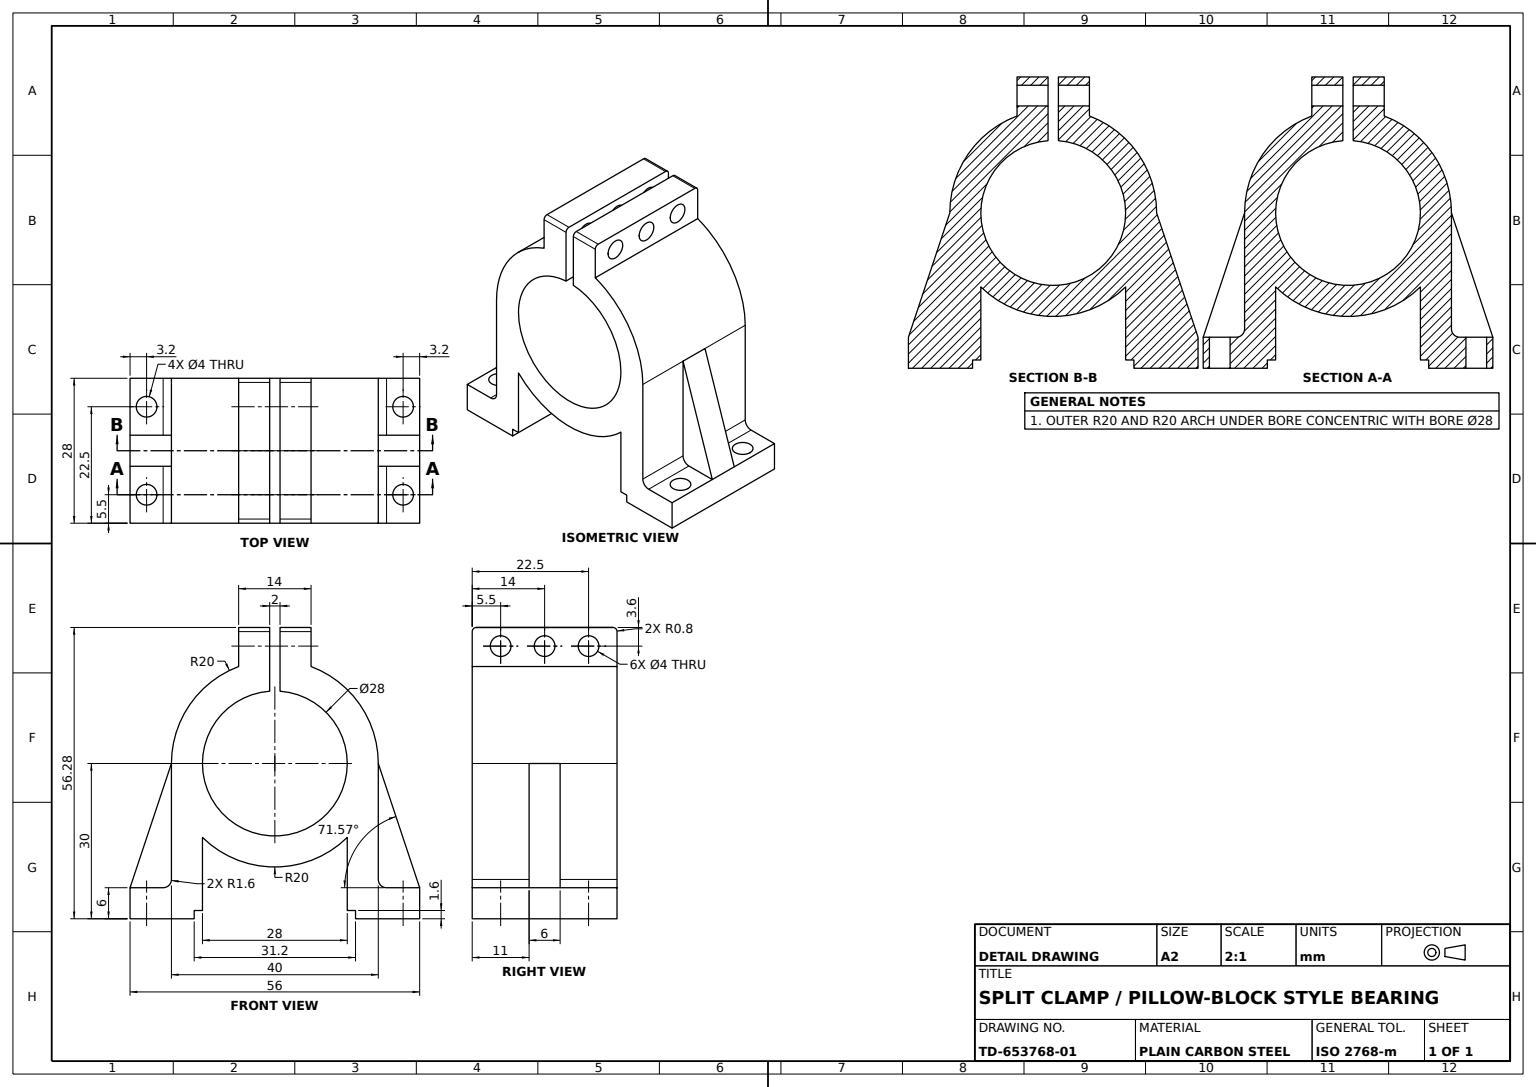
from build123d import *

# Parameters (mm, degrees)
CLAMP_BODY_DEPTH             = 14
CLAMP_BORE_SKETCH_R          = 14
CLAMP_BORE_DEPTH             = 96
CLAMP_LUGS_DEPTH             = 28
SPLIT_SLOT_2MM_DEPTH         = 52
BODY_FILLET_R1_6_A_R         = 1.6
BODY_FILLET_R1_6_B_R         = 1.6
CLAMP_SCREW_HOLES_SKETCH_R   = 2
CLAMP_SCREW_HOLES_3X_DEPTH   = 52
SUPPORT_RIB_1_REACH          = 61.228
SUPPORT_RIB_1_SKETCH_WALL_W  = 145.754223634
SUPPORT_RIB_1_SKETCH_WALL_H  = 6
SUPPORT_RIB_2_REACH          = 61.228
SUPPORT_RIB_2_SKETCH_WALL_W  = 145.754223634
SUPPORT_RIB_2_SKETCH_WALL_H  = 6
BASE_MOUNTING_HOLES_SKETCH_R = 2
BASE_MOUNTING_HOLES_4X_DEPTH = 52
LUG_FILLET_R0_8_A_R          = 0.8
LUG_FILLET_R0_8_B_R          = 0.8
LUG_FILLET_R0_8_C_R          = 0.8
LUG_FILLET_R0_8_D_R          = 0.8


with BuildPart() as part:
    # Clamp Body Profile → Clamp Body (new, symmetric)
    with BuildSketch(Plane.XY):
        with BuildLine():
            Line((20, 24), (20, 0))
            Line((20, 0), (28, 0))
            Line((28, 0), (28, -6))
            Line((28, -6), (15.6, -6))
            Line((15.6, -6), (15.6, -4.4))
            Line((15.6, -4.4), (14, -4.4))
            Line((14, -4.4), (14, 9.717143143))
            ThreePointArc((14, 9.717143143), (0, 4), (-14, 9.717143143))
            Line((-14, 9.717143143), (-14, -4.4))
            Line((-14, -4.4), (-15.6, -4.4))
            Line((-15.6, -4.4), (-15.6, -6))
            Line((-15.6, -6), (-28, -6))
            Line((-28, -6), (-28, 0))
            Line((-28, 0), (-20, 0))
            Line((-20, 0), (-20, 24))
            ThreePointArc((-20, 24), (0, 44), (20, 24))
        make_face()
    extrude(amount=CLAMP_BODY_DEPTH, both=True)

    # Clamp Bore Sketch → Clamp Bore (cut)
    with BuildSketch(Plane.XY.offset(14)):
        with Locations((0, 24)):
            Circle(CLAMP_BORE_SKETCH_R)
    extrude(amount=-CLAMP_BORE_DEPTH, mode=Mode.SUBTRACT)

    # Clamp Lugs Sketch → Clamp Lugs (add)
    with BuildSketch(Plane.XY.offset(14)):
        Polygon((0, 38), (7, 38), (7, 42.734993995), (7, 50.278784028), (-7, 50.278784028), (-7, 38), align=None)
    extrude(amount=-CLAMP_LUGS_DEPTH)

    # Split Slot Sketch → Split Slot 2mm (cut)
    with BuildSketch(Plane.XY.offset(14)):
        Polygon((-1, 37.964240044), (-1, 37.406271495), (1, 37.406271495), (1, 38), (1, 50.278784028), (-1, 50.278784028), align=None)
    extrude(amount=-SPLIT_SLOT_2MM_DEPTH, mode=Mode.SUBTRACT)

    # Body Fillet R1.6 A
    body_fillet_r1_6_a_edges = [part.edges().sort_by_distance(p)[0] for p in [
        (20, 0, 0),
    ]]
    fillet(body_fillet_r1_6_a_edges, radius=BODY_FILLET_R1_6_A_R)

    # Body Fillet R1.6 B
    body_fillet_r1_6_b_edges = [part.edges().sort_by_distance(p)[0] for p in [
        (-20, 0, 0),
    ]]
    fillet(body_fillet_r1_6_b_edges, radius=BODY_FILLET_R1_6_B_R)

    # Clamp Screw Holes Sketch → Clamp Screw Holes 3x (cut)
    with BuildSketch(Plane(origin=(7, 0, 0), x_dir=(0, 0, -1), z_dir=(1, 0, 0))):
        with Locations((8.5, 46.678784028)):
            Circle(CLAMP_SCREW_HOLES_SKETCH_R)
        with Locations((-8.5, 46.678784028)):
            Circle(CLAMP_SCREW_HOLES_SKETCH_R)
        with Locations((0, 46.678784028)):
            Circle(CLAMP_SCREW_HOLES_SKETCH_R)
    extrude(amount=-CLAMP_SCREW_HOLES_3X_DEPTH, mode=Mode.SUBTRACT)

    # Support Rib 1 Sketch wall → Support Rib 1 (add, up to next)
    with BuildSketch(Plane(origin=(24, 12, 0), x_dir=(-0.316227766017, 0.948683298051, 0), z_dir=(-0.948683298051, -0.316227766017, 0)), mode=Mode.PRIVATE) as support_rib_1_sk1:
        Rectangle(SUPPORT_RIB_1_SKETCH_WALL_W, SUPPORT_RIB_1_SKETCH_WALL_H)
    support_rib_1_tool1 = extrude(support_rib_1_sk1.sketch, amount=SUPPORT_RIB_1_REACH, mode=Mode.PRIVATE) - part.part
    add(support_rib_1_tool1.solids().sort_by_distance((24, 12, 0))[0])

    # Support Rib 2 Sketch wall → Support Rib 2 (add, up to next)
    with BuildSketch(Plane(origin=(-24, 12, 0), x_dir=(-0.316227766017, -0.948683298051, 0), z_dir=(0.948683298051, -0.316227766017, 0)), mode=Mode.PRIVATE) as support_rib_2_sk1:
        Rectangle(SUPPORT_RIB_2_SKETCH_WALL_W, SUPPORT_RIB_2_SKETCH_WALL_H)
    support_rib_2_tool1 = extrude(support_rib_2_sk1.sketch, amount=SUPPORT_RIB_2_REACH, mode=Mode.PRIVATE) - part.part
    add(support_rib_2_tool1.solids().sort_by_distance((-24, 12, 0))[0])

    # Base Mounting Holes Sketch → Base Mounting Holes 4x (cut)
    with BuildSketch(Plane(origin=(0, 0, 0), x_dir=(1, 0, 0), z_dir=(0, 1, 0))):
        with Locations(Location((24.8, 8.5, 0), (0, 0, 180))):
            Circle(BASE_MOUNTING_HOLES_SKETCH_R)
        with Locations(Location((24.8, -8.5, 0), (0, 0, 180))):
            Circle(BASE_MOUNTING_HOLES_SKETCH_R)
        with Locations(Location((-24.8, 8.5, 0), (0, 0, 180))):
            Circle(BASE_MOUNTING_HOLES_SKETCH_R)
        with Locations(Location((-24.8, -8.5, 0), (0, 0, 180))):
            Circle(BASE_MOUNTING_HOLES_SKETCH_R)
    extrude(amount=-BASE_MOUNTING_HOLES_4X_DEPTH, mode=Mode.SUBTRACT)

    # Lug Fillet R0.8 A
    lug_fillet_r0_8_a_edges = [part.edges().sort_by_distance(p)[0] for p in [
        (4, 50.278784028, 14),
    ]]
    fillet(lug_fillet_r0_8_a_edges, radius=LUG_FILLET_R0_8_A_R)

    # Lug Fillet R0.8 B
    lug_fillet_r0_8_b_edges = [part.edges().sort_by_distance(p)[0] for p in [
        (-4, 50.278784028, 14),
    ]]
    fillet(lug_fillet_r0_8_b_edges, radius=LUG_FILLET_R0_8_B_R)

    # Lug Fillet R0.8 C
    lug_fillet_r0_8_c_edges = [part.edges().sort_by_distance(p)[0] for p in [
        (-4, 50.278784028, -14),
    ]]
    fillet(lug_fillet_r0_8_c_edges, radius=LUG_FILLET_R0_8_C_R)

    # Lug Fillet R0.8 D
    lug_fillet_r0_8_d_edges = [part.edges().sort_by_distance(p)[0] for p in [
        (4, 50.278784028, -14),
    ]]
    fillet(lug_fillet_r0_8_d_edges, radius=LUG_FILLET_R0_8_D_R)


solid = part.part
